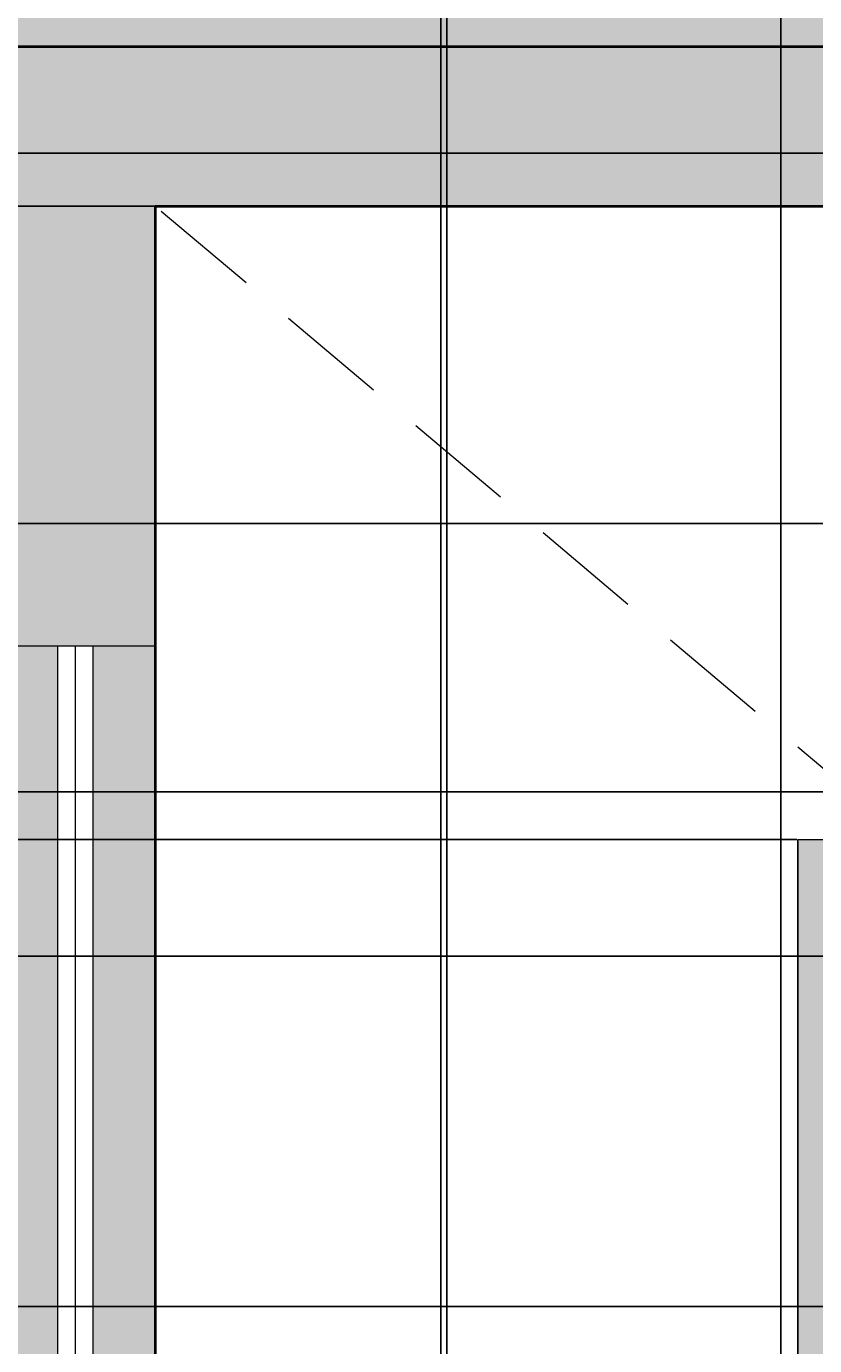
# Model space of a CAD drawing. Units: inches. Extents: x 818 to 1898, y 976 to 2364.
# Tile 72 of 96: x 1260 to 1305, y 1980 to 2054. Entities that reach past the tile are written whole.
import ezdxf

# ---------------------------------------------------------------- set-up
doc = ezdxf.new("R2010")
doc.units = ezdxf.units.IN
doc.header["$LTSCALE"] = 5
doc.header["$MEASUREMENT"] = 0
doc.linetypes.add('HIDDEN', pattern=[0.375, 0.25, -0.125])
for name, color, linetype, lineweight in [('A-ANNO-DIMS', 2, 'Continuous', 18), ('A-FLOR-OVHD', 8, 'HIDDEN', 13), ('A-FURN', 8, 'Continuous', 18), ('A-FURN-PATT', 8, 'Continuous', 9), ('A-GLAZ', 4, 'Continuous', 18), ('A-WALL', 7, 'Continuous', 40)]:
    doc.layers.add(name, color=color, linetype=linetype, lineweight=lineweight)
for name, color, linetype, lineweight, true_color in [('A-GLAZ-PATT', 141, 'Continuous', 9, 0xadddf7), ('A-WALL-PATT', 251, 'Continuous', 13, 0x636466), ('L-PLNT-PATT', 114, 'Continuous', 9, 0x139b48)]:
    doc.layers.add(name, color=color, linetype=linetype, lineweight=lineweight, true_color=true_color)
doc.styles.get("Standard").update_dxf_attribs({"font": 'arial.ttf'})
doc.dimstyles.get("Standard").update_dxf_attribs({"dimtxt": 0.18, "dimasz": 0.18, "dimexe": 0.18, "dimexo": 0.0625, "dimgap": 0.09, "dimtad": 0, "dimtih": 1, "dimtoh": 1, "dimdec": 4, "dimzin": 0, "dimdsep": 46, "dimtxsty": 'Standard', "dimcen": 0.09, "dimadec": 0, "dimazin": 0, "dimtfac": 1, "dimtdec": 4, "dimtofl": 0, "dimtmove": 0, "dimatfit": 3, "dimfxl": 1, "dimtolj": 1, "dimtzin": 0, "dimarcsym": 0})

# ---------------------------------------------------------------- blocks, each defined once
blk = doc.blocks.new('*D61')
at = {"layer": 'A-ANNO-DIMS', "color": 0, "lineweight": -2, "ltscale": 5, "transparency": 16777216}
for p, q in [((1071.725, 1203.027), (1071.725, 2363.873)), ((1071.905, 2363.693), (1250.936, 2363.693)), ((1430.545, 2363.693), (1251.514, 2363.693)), ((1430.725, 1203.027), (1430.725, 2363.873))]:
    blk.add_line(p, q, dxfattribs=at)
at = {"layer": 'A-ANNO-DIMS', "color": 0, "ltscale": 5, "transparency": 16777216}
for points in [[(1071.905, 2363.723), (1071.905, 2363.663), (1071.725, 2363.693)], [(1430.545, 2363.723), (1430.545, 2363.663), (1430.725, 2363.693)]]:
    blk.add_solid(points, dxfattribs=at)
at = {"layer": 'Defpoints', "color": 0, "ltscale": 5, "transparency": 16777216}
for p in [(1430.725, 2363.693), (1071.725, 1202.964), (1430.725, 1202.964)]:
    blk.add_point(p, dxfattribs=at)
at = {"layer": 'A-ANNO-DIMS', "color": 0, "ltscale": 5, "transparency": 16777216, "insert": (1251.225, 2363.693), "char_height": 0.18, "attachment_point": 5}
blk.add_mtext('\\A1;359', dxfattribs=at)
blk = doc.blocks.new('*D64')
at = {"layer": 'A-ANNO-DIMS', "color": 0, "lineweight": -2, "ltscale": 5, "transparency": 16777216}
for p, q in [((1197.725, 1501.141), (1197.725, 2363.873)), ((1197.905, 2363.693), (1313.935, 2363.693)), ((1430.545, 2363.693), (1314.516, 2363.693)), ((1430.725, 1501.141), (1430.725, 2363.873))]:
    blk.add_line(p, q, dxfattribs=at)
at = {"layer": 'A-ANNO-DIMS', "color": 0, "ltscale": 5, "transparency": 16777216}
for points in [[(1197.905, 2363.723), (1197.905, 2363.663), (1197.725, 2363.693)], [(1430.545, 2363.723), (1430.545, 2363.663), (1430.725, 2363.693)]]:
    blk.add_solid(points, dxfattribs=at)
at = {"layer": 'Defpoints', "color": 0, "ltscale": 5, "transparency": 16777216}
for p in [(1430.725, 2363.693), (1197.725, 1501.078), (1430.725, 1501.078)]:
    blk.add_point(p, dxfattribs=at)
at = {"layer": 'A-ANNO-DIMS', "color": 0, "ltscale": 5, "transparency": 16777216, "insert": (1314.225, 2363.693), "char_height": 0.18, "attachment_point": 5}
blk.add_mtext('\\A1;233', dxfattribs=at)
blk = doc.blocks.new('*D73')
at = {"layer": 'A-ANNO-DIMS', "color": 0, "lineweight": -2, "ltscale": 5, "transparency": 16777216}
for p, q in [((1590.663, 2011.078), (818.026, 2011.078)), ((818.206, 2010.898), (818.206, 1996.76)), ((818.206, 1982.258), (818.206, 1996.396)), ((1590.663, 1982.078), (818.026, 1982.078))]:
    blk.add_line(p, q, dxfattribs=at)
at = {"layer": 'A-ANNO-DIMS', "color": 0, "ltscale": 5, "transparency": 16777216}
for points in [[(818.176, 2010.898), (818.236, 2010.898), (818.206, 2011.078)], [(818.176, 1982.258), (818.236, 1982.258), (818.206, 1982.078)]]:
    blk.add_solid(points, dxfattribs=at)
at = {"layer": 'Defpoints', "color": 0, "ltscale": 5, "transparency": 16777216}
for p in [(818.206, 2011.078), (1590.725, 2011.078), (1590.725, 1982.078)]:
    blk.add_point(p, dxfattribs=at)
at = {"layer": 'A-ANNO-DIMS', "color": 0, "ltscale": 5, "transparency": 16777216, "insert": (818.206, 1996.578), "char_height": 0.18, "attachment_point": 5}
blk.add_mtext('\\A1;29', dxfattribs=at)
blk = doc.blocks.new('*D85')
at = {"layer": 'A-ANNO-DIMS', "color": 0, "lineweight": -2, "ltscale": 5, "transparency": 16777216}
for p, q in [((1258.788, 2053.078), (1897.916, 2053.078)), ((1897.736, 2052.898), (1897.736, 1876.76)), ((1897.736, 1700.258), (1897.736, 1876.396)), ((1258.788, 1700.078), (1897.916, 1700.078))]:
    blk.add_line(p, q, dxfattribs=at)
at = {"layer": 'A-ANNO-DIMS', "color": 0, "ltscale": 5, "transparency": 16777216}
for points in [[(1897.706, 2052.898), (1897.766, 2052.898), (1897.736, 2053.078)], [(1897.706, 1700.258), (1897.766, 1700.258), (1897.736, 1700.078)]]:
    blk.add_solid(points, dxfattribs=at)
at = {"layer": 'Defpoints', "color": 0, "ltscale": 5, "transparency": 16777216}
for p in [(1258.725, 2053.078), (1897.736, 2053.078), (1258.725, 1700.078)]:
    blk.add_point(p, dxfattribs=at)
at = {"layer": 'A-ANNO-DIMS', "color": 0, "ltscale": 5, "transparency": 16777216, "insert": (1897.736, 1876.578), "char_height": 0.18, "attachment_point": 5}
blk.add_mtext('\\A1;353', dxfattribs=at)
blk = doc.blocks.new('*D86')
at = {"layer": 'A-ANNO-DIMS', "color": 0, "lineweight": -2, "ltscale": 5, "transparency": 16777216}
for p, q in [((1258.725, 2053.141), (1258.725, 2363.873)), ((1258.905, 2363.693), (1486.433, 2363.693)), ((1714.545, 2363.693), (1487.018, 2363.693)), ((1714.725, 2053.141), (1714.725, 2363.873))]:
    blk.add_line(p, q, dxfattribs=at)
at = {"layer": 'A-ANNO-DIMS', "color": 0, "ltscale": 5, "transparency": 16777216}
for points in [[(1258.905, 2363.723), (1258.905, 2363.663), (1258.725, 2363.693)], [(1714.545, 2363.723), (1714.545, 2363.663), (1714.725, 2363.693)]]:
    blk.add_solid(points, dxfattribs=at)
at = {"layer": 'Defpoints', "color": 0, "ltscale": 5, "transparency": 16777216}
for p in [(1714.725, 2363.693), (1258.725, 2053.078), (1714.725, 2053.078)]:
    blk.add_point(p, dxfattribs=at)
at = {"layer": 'A-ANNO-DIMS', "color": 0, "ltscale": 5, "transparency": 16777216, "insert": (1486.725, 2363.693), "char_height": 0.18, "attachment_point": 5}
blk.add_mtext('\\A1;456', dxfattribs=at)
blk = doc.blocks.new('*D96')
at = {"layer": 'A-ANNO-DIMS', "color": 0, "lineweight": -2, "ltscale": 5, "transparency": 16777216}
for p, q in [((1229.647, 1071.118), (1229.647, 2363.873)), ((1229.827, 2363.693), (1256.516, 2363.693)), ((1283.99, 2363.693), (1257.301, 2363.693)), ((1284.17, 1071.118), (1284.17, 2363.873))]:
    blk.add_line(p, q, dxfattribs=at)
at = {"layer": 'A-ANNO-DIMS', "color": 0, "ltscale": 5, "transparency": 16777216}
for points in [[(1229.827, 2363.723), (1229.827, 2363.663), (1229.647, 2363.693)], [(1283.99, 2363.723), (1283.99, 2363.663), (1284.17, 2363.693)]]:
    blk.add_solid(points, dxfattribs=at)
at = {"layer": 'Defpoints', "color": 0, "ltscale": 5, "transparency": 16777216}
for p in [(1284.17, 2363.693), (1229.647, 1071.055), (1284.17, 1071.055)]:
    blk.add_point(p, dxfattribs=at)
at = {"layer": 'A-ANNO-DIMS', "color": 0, "ltscale": 5, "transparency": 16777216, "insert": (1256.909, 2363.693), "char_height": 0.18, "attachment_point": 5}
blk.add_mtext('\\A1;54.52', dxfattribs=at)
blk = doc.blocks.new('*D97')
at = {"layer": 'A-ANNO-DIMS', "color": 0, "lineweight": -2, "ltscale": 5, "transparency": 16777216}
for p, q in [((1284.17, 1071.118), (1284.17, 2363.873)), ((1284.35, 2363.693), (1310.962, 2363.693)), ((1338.361, 2363.693), (1311.749, 2363.693)), ((1338.541, 1071.118), (1338.541, 2363.873))]:
    blk.add_line(p, q, dxfattribs=at)
at = {"layer": 'A-ANNO-DIMS', "color": 0, "ltscale": 5, "transparency": 16777216}
for points in [[(1284.35, 2363.723), (1284.35, 2363.663), (1284.17, 2363.693)], [(1338.361, 2363.723), (1338.361, 2363.663), (1338.541, 2363.693)]]:
    blk.add_solid(points, dxfattribs=at)
at = {"layer": 'Defpoints', "color": 0, "ltscale": 5, "transparency": 16777216}
for p in [(1338.541, 2363.693), (1284.17, 1071.055), (1338.541, 1071.055)]:
    blk.add_point(p, dxfattribs=at)
at = {"layer": 'A-ANNO-DIMS', "color": 0, "ltscale": 5, "transparency": 16777216, "insert": (1311.355, 2363.693), "char_height": 0.18, "attachment_point": 5}
blk.add_mtext('\\A1;54.37', dxfattribs=at)
blk = doc.blocks.new('*D165')
at = {"layer": 'A-ANNO-DIMS', "color": 0, "lineweight": -2, "ltscale": 5, "transparency": 16777216}
for p, q in [((1283.818, 1510.141), (1283.818, 2363.873)), ((1283.998, 2363.693), (1324.088, 2363.693)), ((1364.966, 2363.693), (1324.876, 2363.693)), ((1365.146, 1510.141), (1365.146, 2363.873))]:
    blk.add_line(p, q, dxfattribs=at)
at = {"layer": 'A-ANNO-DIMS', "color": 0, "ltscale": 5, "transparency": 16777216}
for points in [[(1283.998, 2363.723), (1283.998, 2363.663), (1283.818, 2363.693)], [(1364.966, 2363.723), (1364.966, 2363.663), (1365.146, 2363.693)]]:
    blk.add_solid(points, dxfattribs=at)
at = {"layer": 'Defpoints', "color": 0, "ltscale": 5, "transparency": 16777216}
for p in [(1365.146, 2363.693), (1283.818, 1510.078), (1365.146, 1510.078)]:
    blk.add_point(p, dxfattribs=at)
at = {"layer": 'A-ANNO-DIMS', "color": 0, "ltscale": 5, "transparency": 16777216, "insert": (1324.482, 2363.693), "char_height": 0.18, "attachment_point": 5}
blk.add_mtext('\\A1;81.33', dxfattribs=at)
blk = doc.blocks.new('*D207')
at = {"layer": 'A-ANNO-DIMS', "color": 0, "lineweight": -2, "ltscale": 5, "transparency": 16777216}
for p, q in [((1590.663, 2044.078), (818.026, 2044.078)), ((818.206, 2043.898), (818.206, 2027.76)), ((818.206, 2011.258), (818.206, 2027.396)), ((1590.663, 2011.078), (818.026, 2011.078))]:
    blk.add_line(p, q, dxfattribs=at)
at = {"layer": 'A-ANNO-DIMS', "color": 0, "ltscale": 5, "transparency": 16777216}
for points in [[(818.176, 2043.898), (818.236, 2043.898), (818.206, 2044.078)], [(818.176, 2011.258), (818.236, 2011.258), (818.206, 2011.078)]]:
    blk.add_solid(points, dxfattribs=at)
at = {"layer": 'Defpoints', "color": 0, "ltscale": 5, "transparency": 16777216}
for p in [(818.206, 2044.078), (1590.725, 2044.078), (1590.725, 2011.078)]:
    blk.add_point(p, dxfattribs=at)
at = {"layer": 'A-ANNO-DIMS', "color": 0, "ltscale": 5, "transparency": 16777216, "insert": (818.206, 2027.578), "char_height": 0.18, "attachment_point": 5}
blk.add_mtext('\\A1;33', dxfattribs=at)
blk = doc.blocks.new('*D232')
at = {"layer": 'A-ANNO-DIMS', "color": 0, "lineweight": -2, "ltscale": 5, "transparency": 16777216}
for p, q in [((1303.869, 2008.392), (818.026, 2008.392)), ((818.206, 2008.212), (818.206, 1980.898)), ((818.206, 1953.221), (818.206, 1980.534)), ((1303.869, 1953.041), (818.026, 1953.041))]:
    blk.add_line(p, q, dxfattribs=at)
at = {"layer": 'A-ANNO-DIMS', "color": 0, "ltscale": 5, "transparency": 16777216}
for points in [[(818.176, 2008.212), (818.236, 2008.212), (818.206, 2008.392)], [(818.176, 1953.221), (818.236, 1953.221), (818.206, 1953.041)]]:
    blk.add_solid(points, dxfattribs=at)
at = {"layer": 'Defpoints', "color": 0, "ltscale": 5, "transparency": 16777216}
for p in [(818.206, 2008.392), (1303.931, 2008.392), (1303.931, 1953.041)]:
    blk.add_point(p, dxfattribs=at)
at = {"layer": 'A-ANNO-DIMS', "color": 0, "ltscale": 5, "transparency": 16777216, "insert": (818.206, 1980.716), "char_height": 0.18, "attachment_point": 5}
blk.add_mtext('\\A1;55.35', dxfattribs=at)
blk = doc.blocks.new('*D233')
at = {"layer": 'A-ANNO-DIMS', "color": 0, "lineweight": -2, "ltscale": 5, "transparency": 16777216}
for p, q in [((1267.725, 2044.016), (1267.725, 975.663)), ((1303.931, 2008.329), (1303.931, 975.663)), ((1267.905, 975.843), (1285.365, 975.843)), ((1303.751, 975.843), (1286.292, 975.843))]:
    blk.add_line(p, q, dxfattribs=at)
at = {"layer": 'A-ANNO-DIMS', "color": 0, "ltscale": 5, "transparency": 16777216}
for points in [[(1267.905, 975.873), (1267.905, 975.813), (1267.725, 975.843)], [(1303.751, 975.873), (1303.751, 975.813), (1303.931, 975.843)]]:
    blk.add_solid(points, dxfattribs=at)
at = {"layer": 'Defpoints', "color": 0, "ltscale": 5, "transparency": 16777216}
for p in [(1267.725, 2044.078), (1303.931, 2008.392), (1303.931, 975.843)]:
    blk.add_point(p, dxfattribs=at)
at = {"layer": 'A-ANNO-DIMS', "color": 0, "ltscale": 5, "transparency": 16777216, "insert": (1285.828, 975.843), "char_height": 0.18, "attachment_point": 5}
blk.add_mtext('\\A1;36.206', dxfattribs=at)
blk = doc.blocks.new('*D234')
at = {"layer": 'A-ANNO-DIMS', "color": 0, "lineweight": -2, "ltscale": 5, "transparency": 16777216}
for p, q in [((1267.663, 2044.078), (818.026, 2044.078)), ((818.206, 2043.898), (818.206, 2026.417)), ((818.206, 2008.572), (818.206, 2026.053)), ((1303.869, 2008.392), (818.026, 2008.392))]:
    blk.add_line(p, q, dxfattribs=at)
at = {"layer": 'A-ANNO-DIMS', "color": 0, "ltscale": 5, "transparency": 16777216}
for points in [[(818.176, 2043.898), (818.236, 2043.898), (818.206, 2044.078)], [(818.176, 2008.572), (818.236, 2008.572), (818.206, 2008.392)]]:
    blk.add_solid(points, dxfattribs=at)
at = {"layer": 'Defpoints', "color": 0, "ltscale": 5, "transparency": 16777216}
for p in [(818.206, 2044.078), (1267.725, 2044.078), (1303.931, 2008.392)]:
    blk.add_point(p, dxfattribs=at)
at = {"layer": 'A-ANNO-DIMS', "color": 0, "ltscale": 5, "transparency": 16777216, "insert": (818.206, 2026.235), "char_height": 0.18, "attachment_point": 5}
blk.add_mtext('\\A1;35.69', dxfattribs=at)
blk = doc.blocks.new('*D237')
at = {"layer": 'A-ANNO-DIMS', "color": 0, "lineweight": -2, "ltscale": 5, "transparency": 16777216}
for p, q in [((1310.845, 2026.207), (818.026, 2026.207)), ((818.206, 2026.027), (818.206, 2014.198)), ((818.206, 2002.005), (818.206, 2013.834)), ((1314.197, 2001.825), (818.026, 2001.825))]:
    blk.add_line(p, q, dxfattribs=at)
at = {"layer": 'A-ANNO-DIMS', "color": 0, "ltscale": 5, "transparency": 16777216}
for points in [[(818.176, 2026.027), (818.236, 2026.027), (818.206, 2026.207)], [(818.176, 2002.005), (818.236, 2002.005), (818.206, 2001.825)]]:
    blk.add_solid(points, dxfattribs=at)
at = {"layer": 'Defpoints', "color": 0, "ltscale": 5, "transparency": 16777216}
for p in [(1310.908, 2026.207), (818.206, 2001.825), (1314.26, 2001.825)]:
    blk.add_point(p, dxfattribs=at)
at = {"layer": 'A-ANNO-DIMS', "color": 0, "ltscale": 5, "transparency": 16777216, "insert": (818.206, 2014.016), "char_height": 0.18, "attachment_point": 5}
blk.add_mtext('\\A1;24.383', dxfattribs=at)
blk = doc.blocks.new('*D254')
at = {"layer": 'A-ANNO-DIMS', "color": 0, "lineweight": -2, "ltscale": 5, "transparency": 16777216}
for p, q in [((1267.725, 2044.016), (1267.725, 975.663)), ((1330.305, 2044.016), (1330.305, 975.663)), ((1267.905, 975.843), (1298.621, 975.843)), ((1330.125, 975.843), (1299.409, 975.843))]:
    blk.add_line(p, q, dxfattribs=at)
at = {"layer": 'A-ANNO-DIMS', "color": 0, "ltscale": 5, "transparency": 16777216}
for points in [[(1267.905, 975.873), (1267.905, 975.813), (1267.725, 975.843)], [(1330.125, 975.873), (1330.125, 975.813), (1330.305, 975.843)]]:
    blk.add_solid(points, dxfattribs=at)
at = {"layer": 'Defpoints', "color": 0, "ltscale": 5, "transparency": 16777216}
for p in [(1267.725, 2044.078), (1330.305, 2044.078), (1330.305, 975.843)]:
    blk.add_point(p, dxfattribs=at)
at = {"layer": 'A-ANNO-DIMS', "color": 0, "ltscale": 5, "transparency": 16777216, "insert": (1299.015, 975.843), "char_height": 0.18, "attachment_point": 5}
blk.add_mtext('\\A1;62.58', dxfattribs=at)
blk = doc.blocks.new('*D257')
at = {"layer": 'A-ANNO-DIMS', "color": 0, "lineweight": -2, "ltscale": 5, "transparency": 16777216}
for p, q in [((1399.573, 2077.188), (818.026, 2077.188)), ((818.206, 2077.008), (818.206, 2065.314)), ((818.206, 2053.258), (818.206, 2064.953)), ((1399.573, 2053.078), (818.026, 2053.078))]:
    blk.add_line(p, q, dxfattribs=at)
at = {"layer": 'A-ANNO-DIMS', "color": 0, "ltscale": 5, "transparency": 16777216}
for points in [[(818.176, 2077.008), (818.236, 2077.008), (818.206, 2077.188)], [(818.176, 2053.258), (818.236, 2053.258), (818.206, 2053.078)]]:
    blk.add_solid(points, dxfattribs=at)
at = {"layer": 'Defpoints', "color": 0, "ltscale": 5, "transparency": 16777216}
for p in [(818.206, 2077.188), (1399.636, 2077.188), (1399.636, 2053.078)]:
    blk.add_point(p, dxfattribs=at)
at = {"layer": 'A-ANNO-DIMS', "color": 0, "ltscale": 5, "transparency": 16777216, "insert": (818.206, 2065.133), "char_height": 0.18, "attachment_point": 5}
blk.add_mtext('\\A1;24.11', dxfattribs=at)
blk = doc.blocks.new('*D266')
at = {"layer": 'A-ANNO-DIMS', "color": 0, "lineweight": -2, "ltscale": 5, "transparency": 16777216}
for p, q in [((1780.439, 2053.078), (818.026, 2053.078)), ((818.206, 2052.898), (818.206, 2050.26)), ((818.206, 2047.258), (818.206, 2049.896)), ((1780.439, 2047.078), (818.026, 2047.078))]:
    blk.add_line(p, q, dxfattribs=at)
at = {"layer": 'A-ANNO-DIMS', "color": 0, "ltscale": 5, "transparency": 16777216}
for points in [[(818.176, 2052.898), (818.236, 2052.898), (818.206, 2053.078)], [(818.176, 2047.258), (818.236, 2047.258), (818.206, 2047.078)]]:
    blk.add_solid(points, dxfattribs=at)
at = {"layer": 'Defpoints', "color": 0, "ltscale": 5, "transparency": 16777216}
for p in [(1780.502, 2053.078), (818.206, 2047.078), (1780.502, 2047.078)]:
    blk.add_point(p, dxfattribs=at)
at = {"layer": 'A-ANNO-DIMS', "color": 0, "ltscale": 5, "transparency": 16777216, "insert": (818.206, 2050.078), "char_height": 0.18, "attachment_point": 5}
blk.add_mtext('\\A1;6', dxfattribs=at)
blk = doc.blocks.new('*D269')
at = {"layer": 'A-ANNO-DIMS', "color": 0, "lineweight": -2, "ltscale": 5, "transparency": 16777216}
for p, q in [((1246.938, 1534.141), (1246.938, 2363.873)), ((1247.118, 2363.693), (1293.706, 2363.693)), ((1341.079, 2363.693), (1294.491, 2363.693)), ((1341.259, 1534.141), (1341.259, 2363.873))]:
    blk.add_line(p, q, dxfattribs=at)
at = {"layer": 'A-ANNO-DIMS', "color": 0, "ltscale": 5, "transparency": 16777216}
for points in [[(1247.118, 2363.723), (1247.118, 2363.663), (1246.938, 2363.693)], [(1341.079, 2363.723), (1341.079, 2363.663), (1341.259, 2363.693)]]:
    blk.add_solid(points, dxfattribs=at)
at = {"layer": 'Defpoints', "color": 0, "ltscale": 5, "transparency": 16777216}
for p in [(1341.259, 2363.693), (1246.938, 1534.078), (1341.259, 1534.078)]:
    blk.add_point(p, dxfattribs=at)
at = {"layer": 'A-ANNO-DIMS', "color": 0, "ltscale": 5, "transparency": 16777216, "insert": (1294.099, 2363.693), "char_height": 0.18, "attachment_point": 5}
blk.add_mtext('\\A1;94.32', dxfattribs=at)
blk = doc.blocks.new('*D281')
at = {"layer": 'A-ANNO-DIMS', "color": 0, "lineweight": -2, "ltscale": 5, "transparency": 16777216}
for p, q in [((1250.303, 1913.703), (1250.303, 2363.873)), ((1250.483, 2363.693), (1420.121, 2363.693)), ((1590.545, 2363.693), (1420.907, 2363.693)), ((1590.725, 2011.141), (1590.725, 2363.873))]:
    blk.add_line(p, q, dxfattribs=at)
at = {"layer": 'A-ANNO-DIMS', "color": 0, "ltscale": 5, "transparency": 16777216}
for points in [[(1250.483, 2363.723), (1250.483, 2363.663), (1250.303, 2363.693)], [(1590.545, 2363.723), (1590.545, 2363.663), (1590.725, 2363.693)]]:
    blk.add_solid(points, dxfattribs=at)
at = {"layer": 'Defpoints', "color": 0, "ltscale": 5, "transparency": 16777216}
for p in [(1590.725, 2363.693), (1590.725, 2011.078), (1250.303, 1913.64)]:
    blk.add_point(p, dxfattribs=at)
at = {"layer": 'A-ANNO-DIMS', "color": 0, "ltscale": 5, "transparency": 16777216, "insert": (1420.514, 2363.693), "char_height": 0.18, "attachment_point": 5}
blk.add_mtext('\\A1;340.4', dxfattribs=at)
blk = doc.blocks.new('*D290')
at = {"layer": 'A-ANNO-DIMS', "color": 0, "lineweight": -2, "ltscale": 5, "transparency": 16777216}
for p, q in [((1302.983, 1599.435), (1302.983, 2363.873)), ((1303.163, 2363.693), (1310.57, 2363.693)), ((1318.713, 2363.693), (1311.306, 2363.693)), ((1318.893, 1607.833), (1318.893, 2363.873))]:
    blk.add_line(p, q, dxfattribs=at)
at = {"layer": 'A-ANNO-DIMS', "color": 0, "ltscale": 5, "transparency": 16777216}
for points in [[(1303.163, 2363.723), (1303.163, 2363.663), (1302.983, 2363.693)], [(1318.713, 2363.723), (1318.713, 2363.663), (1318.893, 2363.693)]]:
    blk.add_solid(points, dxfattribs=at)
at = {"layer": 'Defpoints', "color": 0, "ltscale": 5, "transparency": 16777216}
for p in [(1318.893, 2363.693), (1318.893, 1607.771), (1302.983, 1599.372)]:
    blk.add_point(p, dxfattribs=at)
at = {"layer": 'A-ANNO-DIMS', "color": 0, "ltscale": 5, "transparency": 16777216, "insert": (1310.938, 2363.693), "char_height": 0.18, "attachment_point": 5}
blk.add_mtext('\\A1;15.91', dxfattribs=at)

msp = doc.modelspace()

# ---------------------------------------------------------------- hatches: boundary and pattern name
at = {"layer": 'A-FURN-PATT', "ltscale": 5}
h = msp.add_hatch(color=256, dxfattribs=at)
h.dxf.hatch_style = 1
h.paths.add_polyline_path([(1341.9997, 1981.5338), (1317.9034, 2001.8247), (1314.2595, 2001.8247), (1314.2595, 2004.893), (1310.1046, 2008.3917), (1303.9314, 2008.3917), (1303.9314, 1953.0408), (1308.1629, 1953.0408), (1314.2595, 1958.1746), (1314.2595, 1959.6079), (1315.9616, 1959.6079)])
h.paths.add_polyline_path([(1341.9997, 1981.5338), (1315.9616, 1959.6079), (1336.7936, 1959.6079), (1336.7936, 1953.0408), (1345.3966, 1953.0408), (1345.3966, 1959.6079), (1368.0379, 1959.6079)])
h.paths.add_polyline_path([(1402.518, 2008.3917), (1398.8475, 2008.3917), (1398.8475, 2001.8247), (1376.3134, 2001.8247), (1376.3134, 2008.3917), (1373.8948, 2008.3917), (1367.9307, 2003.3695), (1367.9307, 2001.8247), (1366.0961, 2001.8247), (1341.9997, 1981.5338), (1368.0379, 1959.6079), (1375.8366, 1953.0408), (1376.3134, 1953.0408), (1376.3134, 1959.6079), (1398.8475, 1959.6079), (1398.8475, 1953.0408), (1402.518, 1953.0408)])
h.paths.add_polyline_path([(1366.0961, 2001.8247), (1345.3966, 2001.8247), (1345.3966, 2008.3917), (1336.7936, 2008.3917), (1336.7936, 2001.8247), (1317.9034, 2001.8247), (1341.9997, 1981.5338)])
h.paths.add_polyline_path([(1336.7936, 1959.6079), (1315.9616, 1959.6079), (1314.2595, 1958.1746), (1314.2595, 1953.0408), (1336.7936, 1953.0408)], flags=17)
h.paths.add_polyline_path([(1367.9307, 1959.6079), (1345.3966, 1959.6079), (1345.3966, 1953.0408), (1367.9307, 1953.0408)], flags=17)
h.paths.add_polyline_path([(1398.8475, 1959.6079), (1376.3134, 1959.6079), (1376.3134, 1953.0408), (1398.8475, 1953.0408)], flags=17)
h.paths.add_polyline_path([(1368.0379, 1959.6079), (1367.9307, 1959.6079), (1367.9307, 1953.0408), (1375.8366, 1953.0408)], flags=17)
h.paths.add_polyline_path([(1314.2595, 1958.1746), (1308.1629, 1953.0408), (1314.2595, 1953.0408)], flags=17)
h.paths.add_polyline_path([(1315.9616, 1959.6079), (1314.2595, 1959.6079), (1314.2595, 1958.1746)], flags=16)
h.paths.add_polyline_path([(1314.2595, 2008.3917), (1310.1046, 2008.3917), (1314.2595, 2004.893)], flags=17)
h.paths.add_polyline_path([(1336.7936, 2008.3917), (1314.2595, 2008.3917), (1314.2595, 2004.893), (1317.9034, 2001.8247), (1336.7936, 2001.8247)], flags=17)
h.paths.add_polyline_path([(1314.2595, 2004.893), (1314.2595, 2001.8247), (1317.9034, 2001.8247)], flags=16)
h.paths.add_polyline_path([(1367.9307, 2008.3917), (1345.3966, 2008.3917), (1345.3966, 2001.8247), (1366.0961, 2001.8247), (1367.9307, 2003.3695)], flags=17)
h.paths.add_polyline_path([(1398.8475, 2008.3917), (1376.3134, 2008.3917), (1376.3134, 2001.8247), (1398.8475, 2001.8247)], flags=17)
h.paths.add_polyline_path([(1373.8948, 2008.3917), (1367.9307, 2008.3917), (1367.9307, 2003.3695)], flags=17)
h.paths.add_polyline_path([(1367.9307, 2003.3695), (1366.0961, 2001.8247), (1367.9307, 2001.8247)], flags=16)
h.paths.add_polyline_path([(1546.1595, 2044.0782), (1451.7698, 2044.0782), (1451.7698, 2020.0782), (1546.1595, 2020.0782)])
h.paths.add_polyline_path([(1492.0729, 2040.001, 0.431429), (1491.8238, 2040.251), (1491.3087, 2040.251, 0.415217), (1491.0729, 2040.001)], flags=16)
h.paths.add_polyline_path([(1481.8346, 2039.6036), (1511.886, 2039.6036), (1511.886, 2024.9917), (1481.8346, 2024.9917)], flags=16)
h.paths.add_polyline_path([(1491.0729, 2039.4857), (1491.0729, 2039.501), (1492.0729, 2039.501, -0.4117484), (1491.8401, 2039.251), (1491.8229, 2039.251), (1491.8229, 2039.2509, 0.4325918), (1492.0729, 2039.501), (1491.0729, 2039.501, 0.432604), (1491.3229, 2039.2509), (1491.3229, 2039.251), (1491.325, 2039.251, -0.4165823)], flags=0)
h.paths.add_polyline_path([(1485.3701, 2030.9622), (1485.3701, 2034.3556, -0.4142136), (1488.3701, 2037.3556), (1490.3421, 2037.3556, -0.0779193), (1491.0729, 2038.751), (1495.0729, 2038.751, -0.3148679), (1496.07, 2037.1201, -0.3016609), (1497.9049, 2034.3556), (1497.9049, 2030.9622, -0.4142136), (1494.9049, 2027.9622), (1488.3701, 2027.9622, -0.4142136)], flags=0)
h.paths.add_polyline_path([(1490.3229, 2035.751, 0.2655648), (1491.3229, 2036.751), (1491.3229, 2037.126), (1491.0729, 2037.126, -0.7914183), (1490.5434, 2037.251, -0.7914183), (1491.0729, 2037.376), (1491.3229, 2037.376), (1491.3229, 2037.751), (1492.0729, 2037.751), (1492.0729, 2037.376), (1492.3229, 2037.376, -0.7914183), (1492.8524, 2037.251, -0.7914183), (1492.3229, 2037.126), (1492.1491, 2037.126, -0.0866263), (1492.5376, 2036.0294, 0.1070481), (1493.0729, 2035.751), (1490.3229, 2035.751)], flags=0)
h.paths.add_polyline_path([(1491.9774, 2037.251, -1), (1491.4184, 2037.251, -1)], flags=0)
h.paths.add_polyline_path([(1500.0743, 2028.6045), (1500.0743, 2029.4074), (1510.8414, 2029.4074), (1510.8414, 2028.6045)], flags=0)
h.paths.add_polyline_path([(1500.0743, 2030.5314), (1500.0743, 2031.3342), (1510.8414, 2031.3342), (1510.8414, 2030.5314)], flags=0)
h.paths.add_polyline_path([(1500.0743, 2032.94), (1500.0743, 2033.7428), (1510.8414, 2033.7428), (1510.8414, 2032.94)], flags=0)
h.paths.add_polyline_path([(1500.0743, 2035.7499), (1500.0743, 2036.5528), (1510.8414, 2036.5528), (1510.8414, 2035.7499)], flags=0)
h.paths.add_polyline_path([(1590.7251, 2044.0782), (1576.1595, 2044.0782), (1576.1595, 2020.0782), (1590.7251, 2020.0782)])
h.paths.add_polyline_path([(1668.4429, 2044.0782), (1599.7252, 2044.0782), (1599.7252, 2020.0782), (1668.4429, 2020.0782)])
h.paths.add_polyline_path([(1621.2588, 2040.001, 0.431429), (1621.0097, 2040.251), (1620.4946, 2040.251, 0.415217), (1620.2588, 2040.001)], flags=16)
h.paths.add_polyline_path([(1611.0205, 2024.9917), (1611.0205, 2039.6036), (1641.0719, 2039.6036), (1641.0719, 2024.9917)], flags=16)
h.paths.add_polyline_path([(1620.2588, 2039.4857), (1620.2588, 2039.501), (1621.2588, 2039.501, -0.4117484), (1621.026, 2039.251), (1621.0088, 2039.251), (1621.0088, 2039.2509, 0.4325918), (1621.2588, 2039.501), (1620.2588, 2039.501, 0.432604), (1620.5088, 2039.2509), (1620.5088, 2039.251), (1620.5109, 2039.251, -0.4165823)], flags=0)
h.paths.add_polyline_path([(1614.556, 2030.9622), (1614.556, 2034.3556, -0.4142136), (1617.556, 2037.3556), (1619.528, 2037.3556, -0.0779193), (1620.2588, 2038.751), (1624.2588, 2038.751, -0.3148679), (1625.2559, 2037.1201, -0.3016609), (1627.0908, 2034.3556), (1627.0908, 2030.9622, -0.4142136), (1624.0908, 2027.9622), (1617.556, 2027.9622, -0.4142136)], flags=0)
h.paths.add_polyline_path([(1619.5088, 2035.751, 0.2655648), (1620.5088, 2036.751), (1620.5088, 2037.126), (1620.2588, 2037.126, -0.7914183), (1619.7293, 2037.251, -0.7914183), (1620.2588, 2037.376), (1620.5088, 2037.376), (1620.5088, 2037.751), (1621.2588, 2037.751), (1621.2588, 2037.376), (1621.5088, 2037.376, -0.7914183), (1622.0383, 2037.251, -0.7914183), (1621.5088, 2037.126), (1621.335, 2037.126, -0.0866263), (1621.7235, 2036.0294, 0.1070481), (1622.2588, 2035.751), (1619.5088, 2035.751)], flags=0)
h.paths.add_polyline_path([(1620.6043, 2037.251, -1), (1621.1633, 2037.251, -1)], flags=0)
h.paths.add_polyline_path([(1629.2602, 2028.6045), (1629.2602, 2029.4074), (1640.0273, 2029.4074), (1640.0273, 2028.6045)], flags=0)
h.paths.add_polyline_path([(1629.2602, 2030.5314), (1629.2602, 2031.3342), (1640.0273, 2031.3342), (1640.0273, 2030.5314)], flags=0)
h.paths.add_polyline_path([(1629.2602, 2032.94), (1629.2602, 2033.7428), (1640.0273, 2033.7428), (1640.0273, 2032.94)], flags=0)
h.paths.add_polyline_path([(1629.2602, 2035.7499), (1629.2602, 2036.5528), (1640.0273, 2036.5528), (1640.0273, 2035.7499)], flags=0)
h.paths.add_polyline_path([(1705.7252, 2044.0782), (1698.4429, 2044.0782), (1698.4429, 2020.0782), (1705.7252, 2020.0782)])
h.paths.add_polyline_path([(1705.7252, 1972.0782), (1599.7252, 1972.0782), (1599.7252, 1948.0782), (1705.7252, 1948.0782)])
h.paths.add_polyline_path([(1550.0109, 1979.2444), (1483.5451, 1979.2444), (1483.5451, 1948.6602), (1550.0109, 1948.6602)])
h.paths.add_polyline_path([(1490.2586, 1948.6602), (1488.2586, 1948.6602), (1488.2586, 1941.1742, 0.4142136), (1491.2586, 1938.1742), (1500.7446, 1938.1742, -0.4142136)])
h.paths.add_polyline_path([(1513.2306, 1941.1742), (1513.2306, 1948.6602), (1511.2306, 1948.6602, -0.4142136), (1500.7446, 1938.1742), (1510.2306, 1938.1742, 0.4142136)])
h.paths.add_polyline_path([(1518.778, 1948.6602), (1516.778, 1948.6602), (1516.778, 1941.1742, 0.4142136), (1519.778, 1938.1742), (1529.264, 1938.1742, -0.4142136)])
h.paths.add_polyline_path([(1541.75, 1941.1742), (1541.75, 1948.6602), (1539.75, 1948.6602, -0.4142136), (1529.264, 1938.1742), (1538.75, 1938.1742, 0.4142136)])
h.paths.add_polyline_path([(1590.7251, 1900.0782), (1519.6413, 1900.0782), (1519.6413, 1876.0782), (1590.7251, 1876.0782)])
at = {"layer": 'A-GLAZ-PATT', "ltscale": 5}
h = msp.add_hatch(color=256, dxfattribs=at)
h.dxf.hatch_style = 1
h.paths.add_polyline_path([(1283.8183, 1504.5782), (1206.7252, 1504.5782), (1206.7252, 1501.0782), (1283.8183, 1501.0782)])
h.paths.add_polyline_path([(1283.8183, 1510.0782), (1206.7252, 1510.0782), (1206.7252, 1506.5782), (1283.8183, 1506.5782)])
h.paths.add_polyline_path([(1490.9163, 1355.0782), (1439.7252, 1355.0782), (1439.7252, 1409.0522), (1436.2252, 1409.0522), (1436.2252, 1351.5782), (1490.9163, 1351.5782)])
h.paths.add_polyline_path([(1434.2252, 1409.0522), (1430.7251, 1409.0522), (1430.7251, 1346.0782), (1435.0799, 1346.0782), (1435.0731, 1346.1152), (1435.1501, 1346.0782), (1490.9163, 1346.0782), (1490.9163, 1349.5782), (1434.2252, 1349.5782)])
h.paths.add_polyline_path([(1714.7251, 1545.0782), (1711.2252, 1545.0782), (1711.2252, 1521.0782), (1714.7251, 1521.0782)])
h.paths.add_polyline_path([(1709.2252, 1545.0782), (1705.7252, 1545.0782), (1705.7252, 1521.0782), (1709.2252, 1521.0782)])
h.paths.add_polyline_path([(1714.7251, 1687.0782), (1711.2252, 1687.0782), (1711.2252, 1649.9029), (1714.7251, 1649.9029)])
h.paths.add_polyline_path([(1709.2252, 1687.0782), (1705.7252, 1687.0782), (1705.7252, 1649.9029), (1709.2252, 1649.9029)])
h.paths.add_polyline_path([(1709.2252, 1745.5584), (1705.7252, 1745.5584), (1705.7252, 1717.3178), (1709.2252, 1717.3178)])
h.paths.add_polyline_path([(1714.7251, 1745.5584), (1711.2252, 1745.5584), (1711.2252, 1717.3178), (1714.7251, 1717.3178)])
h.paths.add_polyline_path([(1714.7251, 2014.5114), (1711.2252, 2014.5114), (1711.2252, 1962.0338), (1714.7251, 1962.0338)])
h.paths.add_polyline_path([(1709.2252, 2014.5114), (1705.7252, 2014.5114), (1705.7252, 1962.0338), (1709.2252, 1962.0338)])
h.paths.add_polyline_path([(1538.5155, 2047.5782), (1485.1216, 2047.5782), (1485.1216, 2044.0782), (1538.5155, 2044.0782)])
h.paths.add_polyline_path([(1538.5155, 2053.0782), (1485.1216, 2053.0782), (1485.1216, 2049.5782), (1538.5155, 2049.5782)])
h.paths.add_polyline_path([(1388.0315, 2047.5782), (1330.305, 2047.5782), (1330.305, 2044.0782), (1388.0315, 2044.0782)])
h.paths.add_polyline_path([(1388.0315, 2053.0782), (1330.305, 2053.0782), (1330.305, 2049.5782), (1388.0315, 2049.5782)])
h.paths.add_polyline_path([(1262.2252, 2019.2871), (1258.7251, 2019.2871), (1258.7251, 1928.9218), (1262.2252, 1928.9218)])
h.paths.add_polyline_path([(1267.7251, 2019.2871), (1264.2252, 2019.2871), (1264.2252, 1928.9218), (1267.7251, 1928.9218)])
h.paths.add_polyline_path([(1262.2252, 1862.9652), (1258.7251, 1862.9652), (1258.7251, 1814.9652), (1262.2252, 1814.9652)])
h.paths.add_polyline_path([(1267.7251, 1862.9652), (1264.2252, 1862.9652), (1264.2252, 1814.9652), (1267.7251, 1814.9652)])
h.paths.add_polyline_path([(1262.2252, 1755.3321), (1258.7251, 1755.3321), (1258.7251, 1707.3321), (1262.2252, 1707.3321)])
h.paths.add_polyline_path([(1267.7251, 1755.3321), (1264.2252, 1755.3321), (1264.2252, 1707.3321), (1267.7251, 1707.3321)])
h.paths.add_polyline_path([(1251.9333, 1692.5782), (1206.7252, 1692.5782), (1206.7252, 1687.0782), (1251.9333, 1687.0782)])
h.paths.add_polyline_path([(1251.9333, 1700.0782), (1206.7252, 1700.0782), (1206.7252, 1694.5782), (1251.9333, 1694.5782)])
at = {"layer": 'A-WALL-PATT', "ltscale": 5}
h = msp.add_hatch(color=256, dxfattribs=at)
h.dxf.hatch_style = 1
h.paths.add_polyline_path([(1267.7251, 1928.9218), (1258.7251, 1928.9218), (1258.7251, 1913.6401), (1250.3029, 1913.6401), (1250.3029, 1878.3919), (1258.7251, 1878.3919), (1258.7251, 1862.9652), (1267.7251, 1862.9652)])
h.paths.add_polyline_path([(1267.7251, 1814.9652), (1258.7251, 1814.9652), (1258.7251, 1755.3321), (1267.7251, 1755.3321)])
h.paths.add_polyline_path([(1463.7252, 1696.0782), (1267.7251, 1696.0782), (1267.7251, 1707.3321), (1258.7251, 1707.3321), (1258.7251, 1700.0782), (1251.9333, 1700.0782), (1251.9333, 1687.0782), (1463.7252, 1687.0782)])
h.paths.add_polyline_path([(1714.7251, 1717.3178), (1705.7252, 1717.3178), (1705.7252, 1696.0782), (1599.7252, 1696.0782), (1599.7252, 1790.0782), (1705.7252, 1790.0782), (1705.7252, 1785.6125), (1714.7251, 1785.6125), (1714.7251, 1827.2125), (1705.7252, 1827.2125), (1705.7252, 1802.0782), (1599.7252, 1802.0782), (1599.7252, 1867.0782), (1705.7252, 1867.0782), (1705.7252, 1857.2125), (1714.7251, 1857.2125), (1714.7251, 1930.0316), (1741.8409, 1930.0316), (1741.8409, 1935.0316), (1714.7251, 1935.0316), (1714.7251, 1957.0338), (1741.8409, 1957.0338), (1741.8409, 1962.0338), (1714.7251, 1962.0338), (1705.7252, 1962.0338), (1705.7252, 1948.0782), (1599.7252, 1948.0782), (1599.7252, 1981.0782), (1590.7251, 1981.0782), (1590.7251, 1941.0782), (1620.7252, 1941.0782), (1705.7252, 1941.0782), (1705.7252, 1876.0782), (1599.7252, 1876.0782), (1599.7252, 1911.0782), (1590.7251, 1911.0782), (1590.7251, 1876.0782), (1429.2252, 1876.0782), (1429.2252, 1867.0782), (1511.7252, 1867.0782), (1528.593, 1867.0782), (1595.7252, 1867.0782), (1595.7252, 1773.0782), (1520.7252, 1773.0782), (1520.7252, 1837.5823), (1532.593, 1837.5823), (1532.593, 1867.0782), (1528.593, 1867.0782), (1528.593, 1841.5823), (1511.7252, 1841.5823), (1511.7252, 1744.9714), (1520.7252, 1744.9714), (1520.7252, 1761.0782), (1595.7252, 1761.0782), (1595.7252, 1696.0782), (1520.7252, 1696.0782), (1520.7252, 1716.0454), (1511.7252, 1716.0454), (1511.7252, 1696.0782), (1511.7252, 1687.0782), (1714.7251, 1687.0782)])
h.paths.add_polyline_path([(1714.7251, 2053.0782), (1714.7251, 2081.1881), (1709.7252, 2081.1881), (1709.7252, 2053.0782), (1681.6446, 2053.0782), (1681.6446, 2081.1881), (1676.6446, 2081.1881), (1676.6446, 2053.0782), (1538.5155, 2053.0782), (1538.5155, 2044.0782), (1590.7251, 2044.0782), (1590.7251, 2011.0782), (1599.7252, 2011.0782), (1599.7252, 2044.0782), (1705.7252, 2044.0782), (1705.7252, 2014.5114), (1714.7251, 2014.5114)])
h.paths.add_polyline_path([(1485.1216, 2053.0782), (1422.02, 2053.0782), (1422.02, 2081.1881), (1413.02, 2081.1881), (1413.02, 2053.0782), (1399.6356, 2053.0782), (1399.6356, 2081.1881), (1390.6356, 2081.1881), (1390.6356, 2053.0782), (1388.0315, 2053.0782), (1388.0315, 2044.0782), (1416.2743, 2044.0782), (1485.1216, 2044.0782)])
h.paths.add_polyline_path([(1330.305, 2053.0782), (1258.7251, 2053.0782), (1258.7251, 2019.2871), (1267.7251, 2019.2871), (1267.7251, 2044.0782), (1330.305, 2044.0782)])
h.paths.add_polyline_path([(1258.7251, 2053.0782), (1214.6577, 2053.0782), (1214.6577, 2044.0782), (1258.7251, 2044.0782)])
h.paths.add_polyline_path([(1214.6577, 2053.0782), (1180.349, 2053.0782), (1180.349, 2044.0782), (1214.6577, 2044.0782)])
h.paths.add_polyline_path([(1714.7251, 1639.5782), (1741.8409, 1639.5782), (1741.8409, 1643.5782), (1714.7251, 1643.5782), (1714.7251, 1649.9029), (1705.7252, 1649.9029), (1705.7252, 1600.0782), (1477.7252, 1600.0782), (1477.7252, 1591.0782), (1520.7252, 1591.0782), (1616.7252, 1591.0782), (1616.7252, 1416.6857), (1622.7252, 1416.6857), (1622.7252, 1463.0782), (1624.7252, 1463.0782), (1624.7252, 1467.0782), (1622.7252, 1467.0782), (1622.7252, 1591.0782), (1705.7252, 1591.0782), (1705.7252, 1545.0782), (1714.7251, 1545.0782), (1741.8409, 1545.0782), (1741.8409, 1549.0782), (1714.7251, 1549.0782), (1714.7251, 1593.9175), (1737.8409, 1593.9175), (1737.8409, 1597.9175), (1714.7251, 1597.9175)])
h.paths.add_polyline_path([(1674.9024, 2060.7419), (1714.7045, 2060.7419), (1714.7045, 2073.1061), (1674.9024, 2073.1061)], flags=25)
h.paths.add_polyline_path([(1394.5468, 2061.6618), (1422.2344, 2061.6618), (1422.2344, 2074.0261), (1394.5468, 2074.0261)], flags=24)
at = {"layer": 'L-PLNT-PATT', "ltscale": 5}
h = msp.add_hatch(color=256, dxfattribs=at)
h.dxf.hatch_style = 1
h.paths.add_polyline_path([(1789.7173, 2205.9709), (1083.7252, 2205.9709), (1083.7252, 2083.2623), (1218.1114, 2083.2623), (1218.1114, 2053.0782), (1390.6356, 2053.0782), (1390.6356, 2081.1881), (1399.6356, 2081.1881), (1413.02, 2081.1881), (1422.02, 2081.1881), (1422.02, 2053.0782), (1676.6446, 2053.0782), (1676.6446, 2081.1881), (1714.7251, 2081.1881), (1714.7251, 2081.6235), (1789.7173, 2081.6235)])
h.paths.add_polyline_path([(1388.6037, 2145.2461), (1388.6037, 2122.3767), (1373.4756, 2122.3767), (1373.4756, 2145.2461)], flags=16)
h.paths.add_polyline_path([(1408.6922, 2145.2461), (1423.8203, 2145.2461), (1423.8203, 2122.3767), (1408.6922, 2122.3767)], flags=16)
h.paths.add_polyline_path([(1353.3871, 2155.7839), (1353.3871, 2122.3767), (1338.259, 2122.3767), (1338.259, 2155.7839)], flags=16)
h.paths.add_polyline_path([(1443.9089, 2158.4222), (1459.037, 2158.4222), (1459.037, 2122.3767), (1443.9089, 2122.3767)], flags=16)
h.paths.add_polyline_path([(1318.1705, 2145.2461), (1318.1705, 2122.3767), (1303.0424, 2122.3767), (1303.0424, 2145.2461)], flags=16)
h.paths.add_polyline_path([(1479.1255, 2145.2461), (1494.2536, 2145.2461), (1494.2536, 2122.3767), (1479.1255, 2122.3767)], flags=16)
h.paths.add_polyline_path([(1282.9539, 2145.2461), (1282.9539, 2122.3767), (1267.8258, 2122.3767), (1267.8258, 2145.2461)], flags=16)
h.paths.add_polyline_path([(1514.3421, 2145.2461), (1529.4702, 2145.2461), (1529.4702, 2122.3767), (1514.3421, 2122.3767)], flags=16)
h.paths.add_polyline_path([(1247.7373, 2159.4296), (1247.7373, 2122.3767), (1232.6091, 2122.3767), (1232.6091, 2159.4296)], flags=16)
h.paths.add_polyline_path([(1549.5587, 2156.9246), (1564.6868, 2156.9246), (1564.6868, 2122.3767), (1549.5587, 2122.3767)], flags=16)
h.paths.add_polyline_path([(1212.5206, 2145.2461), (1212.5206, 2122.3767), (1197.3925, 2122.3767), (1197.3925, 2145.2461)], flags=16)
h.paths.add_polyline_path([(1584.7753, 2145.2461), (1599.9034, 2145.2461), (1599.9034, 2122.3767), (1584.7753, 2122.3767)], flags=16)
h.paths.add_polyline_path([(1185.1073, 2104.7786), (1190.6407, 2104.7786), (1185.1073, 2098.2505), (1179.5738, 2104.7786)], flags=16)
h.paths.add_polyline_path([(1619.9919, 2145.2461), (1635.1201, 2145.2461), (1635.1201, 2122.3767), (1619.9919, 2122.3767)], flags=16)
h.paths.add_polyline_path([(1655.2086, 2156.1761), (1670.3367, 2156.1761), (1670.3367, 2122.3767), (1655.2086, 2122.3767)], flags=16)
h.paths.add_polyline_path([(1686.5992, 2145.2461), (1701.7273, 2145.2461), (1701.7273, 2122.3767), (1686.5992, 2122.3767)], flags=16)
h.paths.add_polyline_path([(1715.7616, 2145.2461), (1730.8897, 2145.2461), (1730.8897, 2122.3767), (1715.7616, 2122.3767)], flags=16)
h.paths.add_polyline_path([(1753.1652, 2145.2461), (1776.3312, 2145.2461), (1776.3312, 2115.6891), (1753.1652, 2115.6891)], flags=16)
h.paths.add_polyline_path([(1191.4331, 2146.5159), (1176.7891, 2146.5159), (1176.7891, 2134.1516), (1191.4331, 2134.1516)], flags=24)

# ---------------------------------------------------------------- linework, layer by layer
at = {"layer": 'A-FLOR-OVHD', "ltscale": 5}
msp.add_line((1416.2743, 1918.9894), (1267.7251, 2044.0782), dxfattribs=at)
msp.add_lwpolyline([(1267.7251, 2044.0782), (1416.2743, 2044.0782), (1416.2743, 1918.9894), (1267.7251, 1918.9894)], close=True, dxfattribs=at)
at = {"layer": 'A-FURN'}
msp.add_lwpolyline([(1303.9314, 2008.3917), (1402.518, 2008.3917), (1402.518, 1953.0408), (1303.9314, 1953.0408)], close=True, dxfattribs=at)
at = {"layer": 'A-GLAZ'}
for p, q in [((1267.7251, 2019.2871), (1258.7251, 2019.2871)), ((1262.2252, 2019.2871), (1262.2252, 1928.9218)), ((1263.2252, 2019.2871), (1263.2252, 1928.9218)), ((1264.2252, 2019.2871), (1264.2252, 1928.9218))]:
    msp.add_line(p, q, dxfattribs=at)
at = {"layer": 'A-WALL'}
for p, q in [((1083.7252, 2053.0782), (1390.6356, 2053.0782)), ((1267.7251, 2044.0782), (1267.7251, 1862.9652)), ((1267.7251, 2044.0782), (1590.7251, 2044.0782))]:
    msp.add_line(p, q, dxfattribs=at)

# ---------------------------------------------------------------- dimensions: what is measured, and where the dimension line sits
at = {"layer": 'A-ANNO-DIMS', "ltscale": 5}
for base, p1, p2, override, picture, middle in [((1430.7251, 2363.6929), (1071.7251, 1202.9642), (1430.7251, 1202.9642), {"dimdec": 0, "dimlfac": 1, "dimrnd": 0, "dimzin": 0, "dimdsep": 46, "dimlunit": 2}, '*D61', (1251.2251, 2363.6929)), ((1430.7251, 2363.6929), (1197.7251, 1501.0782), (1430.7251, 1501.0782), {"dimdec": 0, "dimlfac": 1, "dimrnd": 0, "dimzin": 0, "dimdsep": 46, "dimlunit": 2}, '*D64', (1314.2251, 2363.6929)), ((1284.1697, 2363.6929), (1229.6474, 1071.0552), (1284.1697, 1071.0552), {"dimdec": 2, "dimlfac": 1, "dimrnd": 0, "dimzin": 0, "dimdsep": 46, "dimlunit": 2}, '*D96', (1256.9085, 2363.6929)), ((1341.2593, 2363.6929), (1246.9377, 1534.0782), (1341.2593, 1534.0782), {"dimdec": 2, "dimlfac": 1, "dimrnd": 0, "dimzin": 0, "dimdsep": 46, "dimlunit": 2}, '*D269', (1294.0985, 2363.6929)), ((1590.7251, 2363.6929), (1250.3029, 1913.6401), (1590.7251, 2011.0782), {"dimdec": 1, "dimlfac": 1, "dimrnd": 0, "dimzin": 0, "dimdsep": 46, "dimlunit": 2}, '*D281', (1420.514, 2363.6929)), ((1714.7251, 2363.6929), (1258.7251, 2053.0782), (1714.7251, 2053.0782), {"dimdec": 0, "dimlfac": 1, "dimrnd": 0, "dimzin": 0, "dimdsep": 46, "dimlunit": 2}, '*D86', (1486.7251, 2363.6929)), ((1365.1463, 2363.6929), (1283.8183, 1510.0782), (1365.1463, 1510.0782), {"dimdec": 2, "dimlfac": 1, "dimrnd": 0, "dimzin": 0, "dimdsep": 46, "dimlunit": 2}, '*D165', (1324.4823, 2363.6929)), ((1338.5412, 2363.6929), (1284.1697, 1071.0552), (1338.5412, 1071.0552), {"dimdec": 2, "dimlfac": 1, "dimrnd": 0, "dimzin": 0, "dimdsep": 46, "dimlunit": 2}, '*D97', (1311.3554, 2363.6929)), ((1318.8931, 2363.6929), (1302.9835, 1599.3725), (1318.8931, 1607.7707), {"dimdec": 2, "dimlfac": 1, "dimrnd": 0, "dimzin": 0, "dimdsep": 46, "dimlunit": 2}, '*D290', (1310.9383, 2363.6929)), ((1303.9314, 975.8433), (1267.7251, 2044.0782), (1303.9314, 2008.3917), {"dimdec": 3, "dimlfac": 1, "dimrnd": 0, "dimzin": 0, "dimdsep": 46, "dimlunit": 2}, '*D233', (1285.8283, 975.8433)), ((1330.305, 975.8433), (1267.7251, 2044.0782), (1330.305, 2044.0782), {"dimdec": 2, "dimlfac": 1, "dimrnd": 0, "dimzin": 0, "dimdsep": 46, "dimlunit": 2}, '*D254', (1299.0151, 975.8433))]:
    dim = msp.add_linear_dim(base=base, p1=p1, p2=p2, dimstyle='Standard', override=override, dxfattribs=at)
    dim.commit()
    dim.dimension.update_dxf_attribs({"geometry": picture, "text_midpoint": middle})
for base, p1, p2, override, picture, middle in [((818.2059, 2077.1881), (1399.6356, 2053.0782), (1399.6356, 2077.1881), {"dimdec": 2, "dimlfac": 1, "dimrnd": 0, "dimzin": 0, "dimdsep": 46, "dimlunit": 2}, '*D257', (818.2059, 2065.1332)), ((818.2059, 2047.0782), (1780.5019, 2053.0782), (1780.5019, 2047.0782), {"dimdec": 0, "dimlfac": 1, "dimrnd": 0, "dimzin": 0, "dimdsep": 46, "dimlunit": 2}, '*D266', (818.2059, 2050.0782)), ((1897.736, 2053.0782), (1258.7251, 1700.0782), (1258.7251, 2053.0782), {"dimdec": 0, "dimlfac": 1, "dimrnd": 0, "dimzin": 0, "dimdsep": 46, "dimlunit": 2}, '*D85', (1897.736, 1876.5782)), ((818.2059, 2044.0782), (1303.9314, 2008.3917), (1267.7251, 2044.0782), {"dimdec": 2, "dimlfac": 1, "dimrnd": 0, "dimzin": 0, "dimdsep": 46, "dimlunit": 2}, '*D234', (818.2059, 2026.235)), ((818.2059, 2044.0782), (1590.7251, 2011.0782), (1590.7251, 2044.0782), {"dimdec": 0, "dimlfac": 1, "dimrnd": 0, "dimzin": 0, "dimdsep": 46, "dimlunit": 2}, '*D207', (818.2059, 2027.5782)), ((818.2059, 2001.8247), (1310.9077, 2026.2074), (1314.2595, 2001.8247), {"dimdec": 3, "dimlfac": 1, "dimrnd": 0, "dimzin": 0, "dimdsep": 46, "dimlunit": 2}, '*D237', (818.2059, 2014.016)), ((818.2059, 2011.0782), (1590.7251, 1982.0782), (1590.7251, 2011.0782), {"dimdec": 0, "dimlfac": 1, "dimrnd": 0, "dimzin": 0, "dimdsep": 46, "dimlunit": 2}, '*D73', (818.2059, 1996.5782)), ((818.2059, 2008.3917), (1303.9314, 1953.0408), (1303.9314, 2008.3917), {"dimdec": 2, "dimlfac": 1, "dimrnd": 0, "dimzin": 0, "dimdsep": 46, "dimlunit": 2}, '*D232', (818.2059, 1980.7163))]:
    dim = msp.add_linear_dim(base=base, p1=p1, p2=p2, angle=90, dimstyle='Standard', override=override, dxfattribs=at)
    dim.commit()
    dim.dimension.update_dxf_attribs({"geometry": picture, "text_midpoint": middle})

doc.saveas('drawing.dxf')
